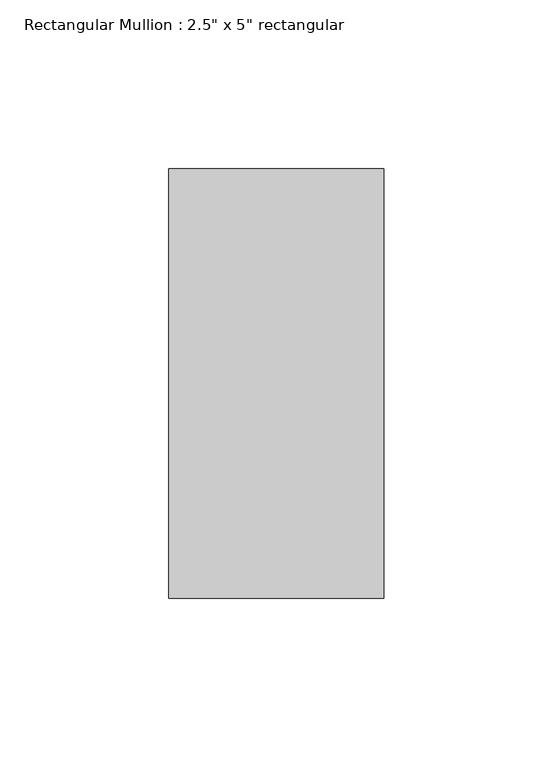
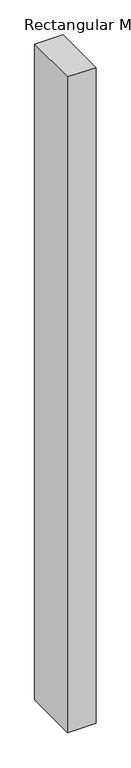
"""IFC4 building model written with IfcOpenShell, lengths in millimetres: member geometry."""

from ifc_helpers import new_model, si_unit, frame, origin, place, context, project, spatial, polyline, outline, extrude, source, transform, mapped, element, save


def member_97f07227(model_context):
    return source(origin(), model_context, "Body", "SweptSolid", [
        extrude(outline(polyline([(31.75, 63.5), (31.75, -63.5), (-31.75, -63.5), (-31.75, 63.5), (31.75, 63.5)])), frame((0.0, 0.0, -1550.2845828), z_axis=(0.0, 0.0, 1.0), x_axis=(1.0, 0.0, 0.0)), (0.0, 0.0, 1.0), 1550.2845828),
    ])


if __name__ == "__main__":
    model = new_model("IFC4")
    model_context = context("Model", 3, world=origin())
    ifc_project = project(units=[si_unit("LENGTHUNIT", "METRE", prefix="MILLI")], contexts=[model_context])
    site = spatial("IfcSite", under=ifc_project)
    building = spatial("IfcBuilding", under=site)
    placement = place(None, origin())
    member_shape = member_97f07227(model_context)
    element("IfcMember", 1, ObjectType="Rectangular Mullion : 2.5\" x 5\" rectangular", at=placement, inside=building, context=model_context, shape_type="MappedRepresentation", body=[
        mapped(member_shape, transform((0.0, 0.0, 0.0), x_axis=(1.0, 0.0, 0.0), y_axis=(0.0, 1.0, 0.0), z_axis=(0.0, 0.0, 1.0))),
    ])
    save(model, "model.ifc")

# Revit data of these elements
# Type "Rectangular Mullion : 2.5\" x 5\" rectangular"
#   built-in parameter 1007304 = 0.416667 (stored number, unit not read)
#   built-in parameter 1007301 = 0.104167 (stored number, unit not read)
#   built-in parameter 1007300 = 0.104167 (stored number, unit not read)
# Element 1 (IfcMember, "Rectangular Mullion : 2.5\" x 5\" rectangular")
#   Materials on its faces: "Aluminum"
# Materials
#   "Aluminum": class "Metal", colour RGB 247 247 247, transparency 0, Description = "Aluminum 6061", Cost = 0
